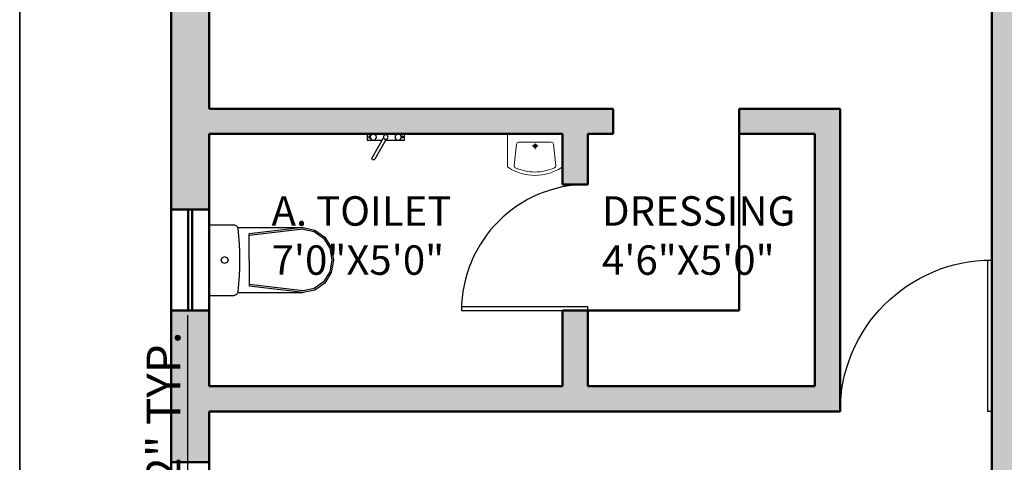
# Model space of a CAD drawing. Units: inches. Extents: x 1986 to 21484, y -1816 to 2016.
# Tile 43 of 85: x 2500 to 2734, y 1616 to 1721. Entities that reach past the tile are written whole.
import ezdxf

# ---------------------------------------------------------------- set-up
doc = ezdxf.new("R2010")
doc.units = ezdxf.units.IN
for name, color, linetype, lineweight in [('A-ANNO-DIMS', 2, 'Continuous', 18), ('A-AREA-IDEN', 3, 'Continuous', 18), ('A-DOOR', 3, 'Continuous', 25), ('A-FLOR-FIXT', 8, 'Continuous', 18), ('A-WALL', 7, 'Continuous', 50), ('A-WALL-PATT', 8, 'Continuous', 13), ('C-PROP', 7, 'Continuous', 35)]:
    doc.layers.add(name, color=color, linetype=linetype, lineweight=lineweight)
doc.layers.add('SANTEH', color=7, linetype='Continuous')
doc.styles.get("Standard").update_dxf_attribs({"font": 'arial.ttf'})
doc.dimstyles.new('ISO-25', dxfattribs={"dimtxt": 8, "dimasz": 2.5, "dimexe": 1.25, "dimexo": 0.625, "dimtad": 1, "dimdec": 1, "dimlunit": 3, "dimtxsty": 'Standard', "dimcen": 2.5, "dimadec": 0, "dimazin": 0, "dimtfac": 1, "dimtdec": 1, "dimtmove": 0, "dimatfit": 3, "dimfxl": 1, "dimarcsym": 0})

# ---------------------------------------------------------------- blocks, each defined once
blk = doc.blocks.new('D2')
for p, q in [((1722.5, 1505.46), (1722.5, 1475.46)), ((1723.5, 1505.46), (1723.5, 1475.46)), ((1722.5, 1475.46), (1723.5, 1475.46))]:
    blk.add_line(p, q)
blk.add_arc((1722.5, 1475.46), 30, 0, 90)
blk = doc.blocks.new('D1')
for p, q in [((1805.96, 1500.36), (1805.96, 1464.36)), ((1806.96, 1500.36), (1806.96, 1464.36)), ((1805.96, 1464.36), (1806.96, 1464.36))]:
    blk.add_line(p, q)
blk.add_arc((1805.96, 1464.36), 36, 0, 90)
blk = doc.blocks.new('WC 2 Symb_109')
at = {"layer": 'SANTEH'}
for p, q in [((0, 0), (0, 380)), ((0, 380), (132.4, 380)), ((153.6, 364.9), (506.8, 364.9)), ((506.3, 364.9), (215.7, 330.9)), ((506.3, 356), (215.7, 322)), ((215.7, 190), (215.7, 330.9)), ((215.7, 190), (215.7, 49.1)), ((506.3, 24), (215.7, 58)), ((153.8, 15.1), (506.8, 15.1)), ((506.3, 15.1), (215.7, 49.1)), ((0, 0), (132.4, 0))]:
    blk.add_line(p, q, dxfattribs=at)
for points in [[(154.6, 360.1), (153.9, 364.1), (152.3, 367.9), (150.2, 371.3), (147.4, 374.3), (144.1, 376.7), (140.5, 378.5), (136.5, 379.6), (132.4, 380)], [(154.6, 19.7), (158.6, 62.1), (161.4, 104.7), (163.1, 147.3), (163.7, 189.9), (163.1, 232.5), (161.4, 275.1), (158.6, 317.7), (154.6, 360.1)], [(506.3, 24), (565.5, 36.6), (615.7, 72.6), (649.2, 126.5), (661, 190), (649.2, 253.5), (615.7, 307.4), (565.5, 343.4), (506.3, 356)], [(506.8, 15.1), (569.2, 28.4), (622.2, 66.3), (657.6, 123.1), (670, 190), (657.6, 256.9), (622.2, 313.7), (569.2, 351.6), (506.8, 364.9)], [(132.4, 0), (136.5, 0.4), (140.4, 1.5), (144.1, 3.2), (147.3, 5.6), (150.1, 8.6), (152.3, 12), (153.8, 15.7), (154.6, 19.7)]]:
    blk.add_lwpolyline(points, dxfattribs=at)
blk.add_lwpolyline([(83.6, 208.5), (70.4, 203.1), (64.9, 190), (70.4, 176.9), (83.6, 171.5), (96.8, 176.9), (102.2, 190), (96.8, 203.1)], close=True, dxfattribs=at)
blk = doc.blocks.new('A$C2EBB240D')
for p, q in [((480, 375.8), (20, 375.8)), ((0, 355.8), (0, 86.6)), ((60.8, 89.8), (82.3, 282.2)), ((250, 300), (102.1, 300)), ((250, 300), (397.9, 300)), ((439.2, 89.8), (417.7, 282.2)), ((500, 355.8), (500, 86.6))]:
    blk.add_line(p, q)
for points in [[(247.3, 238.5), (247.3, 288.9)], [(275.2, 266.4), (219.4, 266.4)]]:
    blk.add_lwpolyline(points)
for centre, radius, start, end in [((20, 355.8), 20, 90, 180), ((480, 355.8), 20, 0, 90), ((102.1, 280), 20, 90, 173.64284), ((247.3, 266.4), 16.7, 90, 270), ((247.3, 266.4), 10, 90, 270), ((247.3, 266.4), 16.7, 270, 90), ((247.3, 266.4), 10, 270, 90), ((397.9, 280), 20, 6.35716, 90), ((80.7, 87.6), 20, 173.64284, 244.97956), ((419.3, 87.6), 20, 295.02044, 6.35716), ((20, 86.6), 20, 180, 237.68921), ((250, 450.3), 450.3, 237.68921, 270), ((250, 450.3), 420.3, 244.97956, 270), ((250, 450.3), 450.3, 270, 302.31079), ((250, 450.3), 420.3, 270, 295.02044), ((480, 86.6), 20, 302.31079, 0)]:
    blk.add_arc(centre, radius, start, end)
blk = doc.blocks.new('Faucet - kit sink top')
at = {"layer": 'SANTEH'}
for p, q in [((-5.5, -0.75), (-5.5, -1.25)), ((-4.94278, -0.75), (-5.5, -0.75)), ((-5.5, -1.25), (-4.94278, -1.25)), ((-0.14775, -1.7441), (3.56698, -8.1782)), ((4.43301, -7.6782), (0.71828, -1.2441)), ((4.94278, -0.75), (5.5, -0.75)), ((5.5, -1.25), (4.94278, -1.25)), ((5.5, -0.75), (5.5, -1.25))]:
    blk.add_line(p, q, dxfattribs=at)
blk.add_lwpolyline([(-0.00587, -2), (-6, -2), (-6, 0), (6, 0), (6, -2), (1.15195, -2)], dxfattribs=at)
for centre, radius in [((-4, -1), 1), ((4, -1), 1), ((0, -1), 0.75)]:
    blk.add_circle(centre, radius, dxfattribs=at)
blk.add_arc((4, -7.9282), 0.5, 210, 30, dxfattribs=at)
blk = doc.blocks.new('*D109')
at = {"layer": 'A-ANNO-DIMS', "color": 0, "lineweight": -2, "transparency": 16777216}
for p, q in [((2540.28, 1510.13), (2540.28, 1650.68)), ((2544.98, 1510.13), (2539.03, 1510.13)), ((2540.28, 1477.15), (2540.28, 1507.63)), ((2544.98, 1474.65), (2539.03, 1474.65))]:
    blk.add_line(p, q, dxfattribs=at)
at = {"layer": 'A-ANNO-DIMS', "color": 0, "transparency": 16777216}
for points in [[(2539.86, 1507.63), (2540.7, 1507.63), (2540.28, 1510.13)], [(2539.86, 1477.15), (2540.7, 1477.15), (2540.28, 1474.65)]]:
    blk.add_solid(points, dxfattribs=at)
at = {"layer": 'Defpoints', "color": 0, "transparency": 16777216}
for p in [(2540.28, 1510.13), (2545.6, 1510.13), (2545.6, 1474.65)]:
    blk.add_point(p, dxfattribs=at)
at = {"layer": 'A-ANNO-DIMS', "color": 0, "transparency": 16777216, "insert": (2535.52, 1581.65), "char_height": 8, "attachment_point": 5, "rotation": 90}
blk.add_mtext('ARMCHAIR 2\'-11 1/2" TYP.', dxfattribs=at)

msp = doc.modelspace()

# ---------------------------------------------------------------- hatches: boundary and pattern name
at = {"layer": 'A-WALL-PATT'}
h = msp.add_hatch(color=256, dxfattribs=at)
h.dxf.hatch_style = 1
h.paths.add_polyline_path([(2545.31, 1843.75), (2665.31, 1843.75), (2665.31, 1852.75), (2536.31, 1852.75), (2536.31, 1765.75), (2545.31, 1765.75)])
h.paths.add_polyline_path([(2545.31, 1723.75), (2536.31, 1723.75), (2536.31, 1675.75), (2545.31, 1675.75), (2545.31, 1693.75), (2629.31, 1693.75), (2629.31, 1681.75), (2635.31, 1681.75), (2635.31, 1693.75), (2641.31, 1693.75), (2641.31, 1699.75), (2545.31, 1699.75)])
h.paths.add_polyline_path([(2545.31, 1651.75), (2536.31, 1651.75), (2536.31, 1615.75), (2545.31, 1615.75), (2545.31, 1627.75), (2695.31, 1627.75), (2695.31, 1699.75), (2671.31, 1699.75), (2671.31, 1693.75), (2689.31, 1693.75), (2689.31, 1633.75), (2635.31, 1633.75), (2635.31, 1651.75), (2629.31, 1651.75), (2629.31, 1633.75), (2545.31, 1633.75)])
h.paths.add_polyline_path([(2545.31, 1573.75), (2536.31, 1573.75), (2536.31, 1528.77), (2545.31, 1528.77)])
h.paths.add_polyline_path([(2545.31, 1486.77), (2536.31, 1486.77), (2536.31, 1441.75), (2545.31, 1441.75)])
h.paths.add_polyline_path([(2545.31, 1399.75), (2536.31, 1399.75), (2536.31, 1258.75), (2545.31, 1258.75)])
h.paths.add_polyline_path([(2609.81, 1387.75), (2581.31, 1387.75), (2581.31, 1378.75), (2609.81, 1378.75)])
h.paths.add_polyline_path([(2677.31, 1387.75), (2651.81, 1387.75), (2651.81, 1378.75), (2668.31, 1378.75), (2668.31, 1354.75), (2677.31, 1354.75)])
h.paths.add_polyline_path([(2842.31, 1387.75), (2833.31, 1387.75), (2713.31, 1387.75), (2713.31, 1381.75), (2833.31, 1381.75), (2833.31, 1363.75), (2842.31, 1363.75)])
h.paths.add_polyline_path([(2842.31, 1339.75), (2833.31, 1339.75), (2833.31, 1321.75), (2737.31, 1321.75), (2737.31, 1351.75), (2731.31, 1351.75), (2731.31, 1315.75), (2833.31, 1315.75), (2833.31, 1303.75), (2842.31, 1303.75)])
h.paths.add_polyline_path([(2677.31, 1312.75), (2668.31, 1312.75), (2668.31, 1189.75), (2677.31, 1189.75)])
h.paths.add_polyline_path([(2677.31, 1147.75), (2668.31, 1147.75), (2668.31, 1114.75), (2683.31, 1114.75), (2683.31, 1123.75), (2677.31, 1123.75)])
h.paths.add_polyline_path([(2842.31, 1147.75), (2833.31, 1147.75), (2833.31, 1123.75), (2725.31, 1123.75), (2725.31, 1114.75), (2842.31, 1114.75)])
h.paths.add_polyline_path([(2842.31, 1261.75), (2833.31, 1261.75), (2833.31, 1189.75), (2842.31, 1189.75)])
h.paths.add_polyline_path([(2842.31, 1441.75), (2833.31, 1441.75), (2833.31, 1423.75), (2842.31, 1423.75)])
h.paths.add_polyline_path([(2842.31, 1495.75), (2833.31, 1495.75), (2833.31, 1477.75), (2842.31, 1477.75)])
h.paths.add_polyline_path([(2737.31, 1852.75), (2707.31, 1852.75), (2707.31, 1843.75), (2731.31, 1843.75), (2731.31, 1573.75), (2737.31, 1573.75)])
h.paths.add_polyline_path([(2719.29, 1802.81), (2719.29, 1755.53), (2727.83, 1755.53), (2727.83, 1802.81)], flags=25)
h.paths.add_polyline_path([(2682.04, 1129.8), (2724.23, 1129.8), (2724.23, 1138.34), (2682.04, 1138.34)], flags=9)
h.paths.add_polyline_path([(2763.84, 1129.8), (2811.12, 1129.8), (2811.12, 1138.34), (2763.84, 1138.34)], flags=25)
h.paths.add_polyline_path([(2759.39, 1682.81), (2810.29, 1682.81), (2810.29, 1709.43), (2759.39, 1709.43)], flags=9)
h.paths.add_polyline_path([(2636.77, 1656.28), (2690.81, 1656.28), (2690.81, 1682.89), (2636.77, 1682.89)], flags=25)
h.paths.add_polyline_path([(2525.6, 1419.09), (2525.6, 1479.38), (2510.65, 1479.38), (2510.65, 1419.09)], flags=9)
h.paths.add_polyline_path([(2860.43, 1418.3), (2860.43, 1487.98), (2845.48, 1487.98), (2845.48, 1418.3)], flags=9)
h.paths.add_polyline_path([(2725.63, 1084.99), (2785.92, 1084.99), (2785.92, 1099.93), (2725.63, 1099.93)], flags=9)
h.paths.add_polyline_path([(2602.46, 1501.1), (2675.15, 1501.1), (2675.15, 1527.71), (2602.46, 1527.71)], flags=9)
h.paths.add_polyline_path([(2571.3, 1320.51), (2625.79, 1320.51), (2625.79, 1347.12), (2571.3, 1347.12)], flags=9)
h.paths.add_polyline_path([(2729.91, 1208.98), (2797.91, 1208.98), (2797.91, 1235.59), (2729.91, 1235.59)], flags=9)
h.paths.add_polyline_path([(2753.97, 1338.54), (2806.8, 1338.54), (2806.8, 1365.15), (2753.97, 1365.15)], flags=9)
h.paths.add_polyline_path([(2605.23, 1760.02), (2661.46, 1760.02), (2661.46, 1786.64), (2605.23, 1786.64)], flags=9)
h.paths.add_polyline_path([(2558.03, 1656.28), (2610.63, 1656.28), (2610.63, 1682.89), (2558.03, 1682.89)], flags=25)
h = msp.add_hatch(color=256, dxfattribs=at)
h.dxf.hatch_style = 1
h.paths.add_polyline_path([(2842.31, 1852.75), (2737.31, 1852.75), (2737.31, 1843.75), (2833.31, 1843.75), (2833.31, 1537.75), (2842.31, 1537.75)])
h.paths.add_polyline_path([(2682.04, 1129.8), (2724.23, 1129.8), (2724.23, 1138.34), (2682.04, 1138.34)], flags=9)
h.paths.add_polyline_path([(2763.84, 1129.8), (2811.12, 1129.8), (2811.12, 1138.34), (2763.84, 1138.34)], flags=9)
h.paths.add_polyline_path([(2719.29, 1802.81), (2719.29, 1755.53), (2727.83, 1755.53), (2727.83, 1802.81)], flags=9)
h.paths.add_polyline_path([(2759.39, 1682.81), (2810.29, 1682.81), (2810.29, 1709.43), (2759.39, 1709.43)], flags=25)
h.paths.add_polyline_path([(2636.77, 1656.28), (2690.81, 1656.28), (2690.81, 1682.89), (2636.77, 1682.89)], flags=9)
h.paths.add_polyline_path([(2525.6, 1419.09), (2525.6, 1479.38), (2510.65, 1479.38), (2510.65, 1419.09)], flags=9)
h.paths.add_polyline_path([(2860.43, 1418.3), (2860.43, 1487.98), (2845.48, 1487.98), (2845.48, 1418.3)], flags=9)
h.paths.add_polyline_path([(2725.63, 1084.99), (2785.92, 1084.99), (2785.92, 1099.93), (2725.63, 1099.93)], flags=9)
h.paths.add_polyline_path([(2602.46, 1501.1), (2675.15, 1501.1), (2675.15, 1527.71), (2602.46, 1527.71)], flags=9)
h.paths.add_polyline_path([(2571.3, 1320.51), (2625.79, 1320.51), (2625.79, 1347.12), (2571.3, 1347.12)], flags=9)
h.paths.add_polyline_path([(2710.58, 1210.46), (2778.57, 1210.46), (2778.57, 1237.07), (2710.58, 1237.07)], flags=9)
h.paths.add_polyline_path([(2753.97, 1338.54), (2806.8, 1338.54), (2806.8, 1365.15), (2753.97, 1365.15)], flags=9)
h.paths.add_polyline_path([(2605.23, 1728.88), (2661.46, 1728.88), (2661.46, 1755.49), (2605.23, 1755.49)], flags=9)
h.paths.add_polyline_path([(2558.03, 1656.28), (2610.63, 1656.28), (2610.63, 1682.89), (2558.03, 1682.89)], flags=9)

# ---------------------------------------------------------------- linework, layer by layer
at = {"layer": 'A-WALL'}
for p, q in [((2536.31, 1258.75), (2536.31, 1852.75)), ((2545.31, 1699.75), (2545.31, 1843.75)), ((2731.31, 1843.75), (2731.31, 1573.75)), ((2545.31, 1699.75), (2641.31, 1699.75)), ((2641.31, 1699.75), (2641.31, 1693.75)), ((2671.31, 1699.75), (2671.31, 1651.75)), ((2671.31, 1699.75), (2695.31, 1699.75)), ((2695.31, 1699.75), (2695.31, 1627.75)), ((2545.31, 1693.75), (2629.31, 1693.75)), ((2545.31, 1633.75), (2545.31, 1693.75)), ((2629.31, 1681.75), (2629.31, 1693.75)), ((2635.31, 1693.75), (2641.31, 1693.75)), ((2635.31, 1681.75), (2635.31, 1693.75)), ((2671.31, 1693.75), (2689.31, 1693.75)), ((2689.31, 1693.75), (2689.31, 1633.75)), ((2629.31, 1681.75), (2635.31, 1681.75)), ((2536.31, 1675.75), (2545.31, 1675.75)), ((2540.31, 1651.75), (2540.31, 1675.75)), ((2541.31, 1651.75), (2541.31, 1675.75)), ((2536.31, 1651.75), (2545.31, 1651.75)), ((2629.31, 1651.75), (2671.31, 1651.75)), ((2629.31, 1633.75), (2629.31, 1651.75)), ((2635.31, 1633.75), (2635.31, 1651.75)), ((2545.31, 1633.75), (2629.31, 1633.75)), ((2635.31, 1633.75), (2689.31, 1633.75)), ((2545.31, 1258.75), (2545.31, 1627.75)), ((2545.31, 1627.75), (2695.31, 1627.75)), ((2536.31, 1615.75), (2545.31, 1615.75))]:
    msp.add_line(p, q, dxfattribs=at)
at = {"layer": 'C-PROP'}
msp.add_lwpolyline([(2500.31, 1900.75), (2860.31, 1900.75), (2860.31, 1066.75), (2500.31, 1066.75)], close=True, dxfattribs=at)

# ---------------------------------------------------------------- block references
at = {"layer": 'A-DOOR', "rotation": 90}
msp.add_blockref('D2', (4110.76, -70.75), dxfattribs=at)
at = {"layer": 'A-DOOR', "xscale": -1}
msp.add_blockref('D1', (4537.27, 163.39), dxfattribs=at)
at = {"layer": 'A-FLOR-FIXT'}
for name, p, xscale, yscale, zscale in [('Faucet - kit sink top', (2587.31, 1693.75), -0.7356136897818673, 0.7356136897818673, 0.7356136897818673), ('A$C2EBB240D', (2629.31, 1683.9), -0.026211548048557, 0.026211548048557, 0.026211548048557)]:
    msp.add_blockref(name, p, dxfattribs=dict(at, xscale=xscale, yscale=yscale, zscale=zscale))
at = {"layer": 'A-FLOR-FIXT', "xscale": -0.0441898926459964, "yscale": 0.0441898926459964, "zscale": 0.0441898926459964, "rotation": 180}
msp.add_blockref('WC 2 Symb_109', (2545.31, 1672.15), dxfattribs=at)

# ---------------------------------------------------------------- texts
at = {"layer": 'A-AREA-IDEN', "char_height": 7, "attachment_point": 1}
for s, insert in [('{\\fTimes New Roman|b0|i0|c0|p18;A. TOILET\\P7\'0"X5\'0"}', (2560.16, 1678.93)), ('{\\fTimes New Roman|b0|i0|c0|p18;DRESSING\\P4\'6"X5\'0"}', (2638.69, 1678.93))]:
    msp.add_mtext_dynamic_manual_height_columns(s, width=105.6127, gutter_width=12.5, heights=[0], dxfattribs=dict(at, insert=insert))

# ---------------------------------------------------------------- dimensions: what is measured, and where the dimension line sits
at = {"layer": 'A-ANNO-DIMS'}
dim = msp.add_linear_dim(base=(2540.28, 1510.13), p1=(2545.6, 1474.65), p2=(2545.6, 1510.13), angle=90, text='ARMCHAIR <> TYP.', dimstyle='ISO-25', override={"dimdec": 1, "dimrnd": 0, "dimzin": 1, "dimlunit": 4, "dimfrac": 2}, dxfattribs=at)
dim.commit()
dim.dimension.update_dxf_attribs({"geometry": '*D109', "text_midpoint": (2535.52, 1581.65)})

doc.saveas('drawing.dxf')
